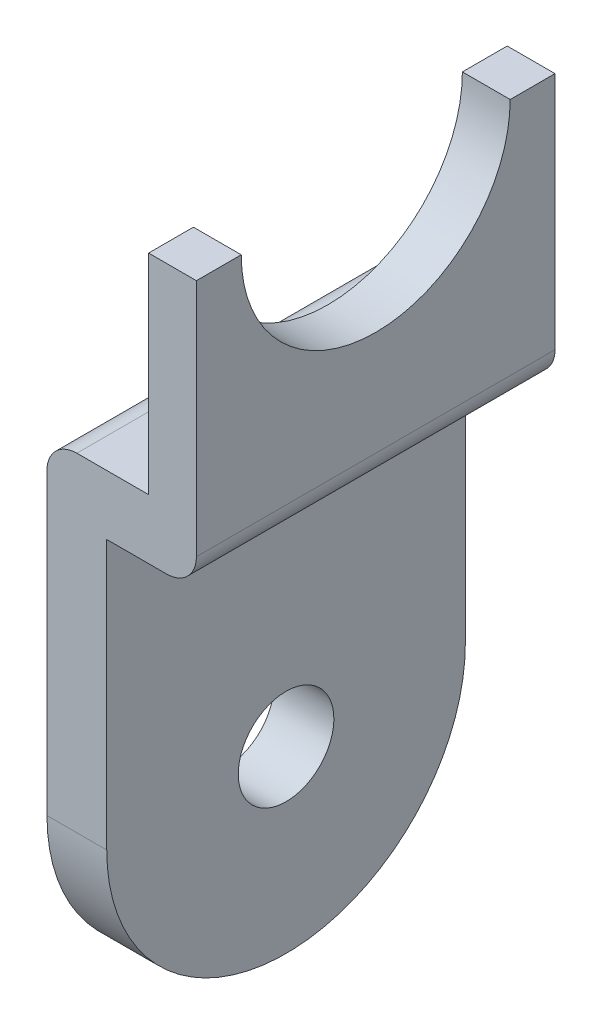
from build123d import *

# Parameters (mm, degrees)
CLIP_BODY_DEPTH      = 6
ROUNDED_TAB_SKETCH_R = 6
ROUNDED_TAB_DEPTH    = 2
SADDLE_CUT_REACH     = 20.708
PIVOT_HOLE_3_2_REACH = 20.276
PIVOT_HOLE_SKETCH_R  = 1.6
EDGE_FILLETS_R1_R    = 1


with BuildPart() as part:
    # Clip Profile Sketch → Clip Body (new, symmetric)
    with BuildSketch(Plane.XY):
        Polygon((0, -11), (0, 0), (3.4, 0), (3.4, 7), (5, 7), (5, -2), (2, -2), (2, -11), align=None)
    extrude(amount=CLIP_BODY_DEPTH, both=True)

    # Rounded Tab Sketch → Rounded Tab (add)
    with BuildSketch(Plane(origin=(2, 0, 0), x_dir=(0, 0, -1), z_dir=(1, 0, 0))):
        with Locations((0, -11)):
            Circle(ROUNDED_TAB_SKETCH_R)
    extrude(amount=-ROUNDED_TAB_DEPTH)

    # Saddle Cut Sketch → Saddle Cut (cut, up to next)
    with BuildSketch(Plane(origin=(5, 0, 0), x_dir=(0, 0, -1), z_dir=(1, 0, 0)), mode=Mode.PRIVATE) as saddle_cut_sk1:
        with BuildLine():
            Line((-4.5, 7), (4.5, 7))
            ThreePointArc((4.5, 7), (0, 2.5), (-4.5, 7))
        make_face()
    saddle_cut_tool1 = extrude(saddle_cut_sk1.sketch, amount=-SADDLE_CUT_REACH, mode=Mode.PRIVATE) & part.part
    add(saddle_cut_tool1.solids().sort_by_distance((5, 5.090141, 0))[0], mode=Mode.SUBTRACT)

    # Pivot Hole Sketch → Pivot Hole Ø3.2 (cut, up to next)
    with BuildSketch(Plane(origin=(2, 0, 0), x_dir=(0, 0, -1), z_dir=(1, 0, 0)), mode=Mode.PRIVATE) as pivot_hole_3_2_sk1:
        with Locations(Location((0, -11, 0), (0, 0, 90))):
            Circle(PIVOT_HOLE_SKETCH_R)
    pivot_hole_3_2_tool1 = extrude(pivot_hole_3_2_sk1.sketch, amount=-PIVOT_HOLE_3_2_REACH, mode=Mode.PRIVATE) & part.part
    add(pivot_hole_3_2_tool1.solids().sort_by_distance((2, -11, 0))[0], mode=Mode.SUBTRACT)

    # Edge Fillets R1
    edge_fillets_r1_edges = [part.edges().sort_by_distance(p)[0] for p in [
        (0, 0, 0),
        (5, -2, 0),
    ]]
    fillet(edge_fillets_r1_edges, radius=EDGE_FILLETS_R1_R)


solid = part.part
